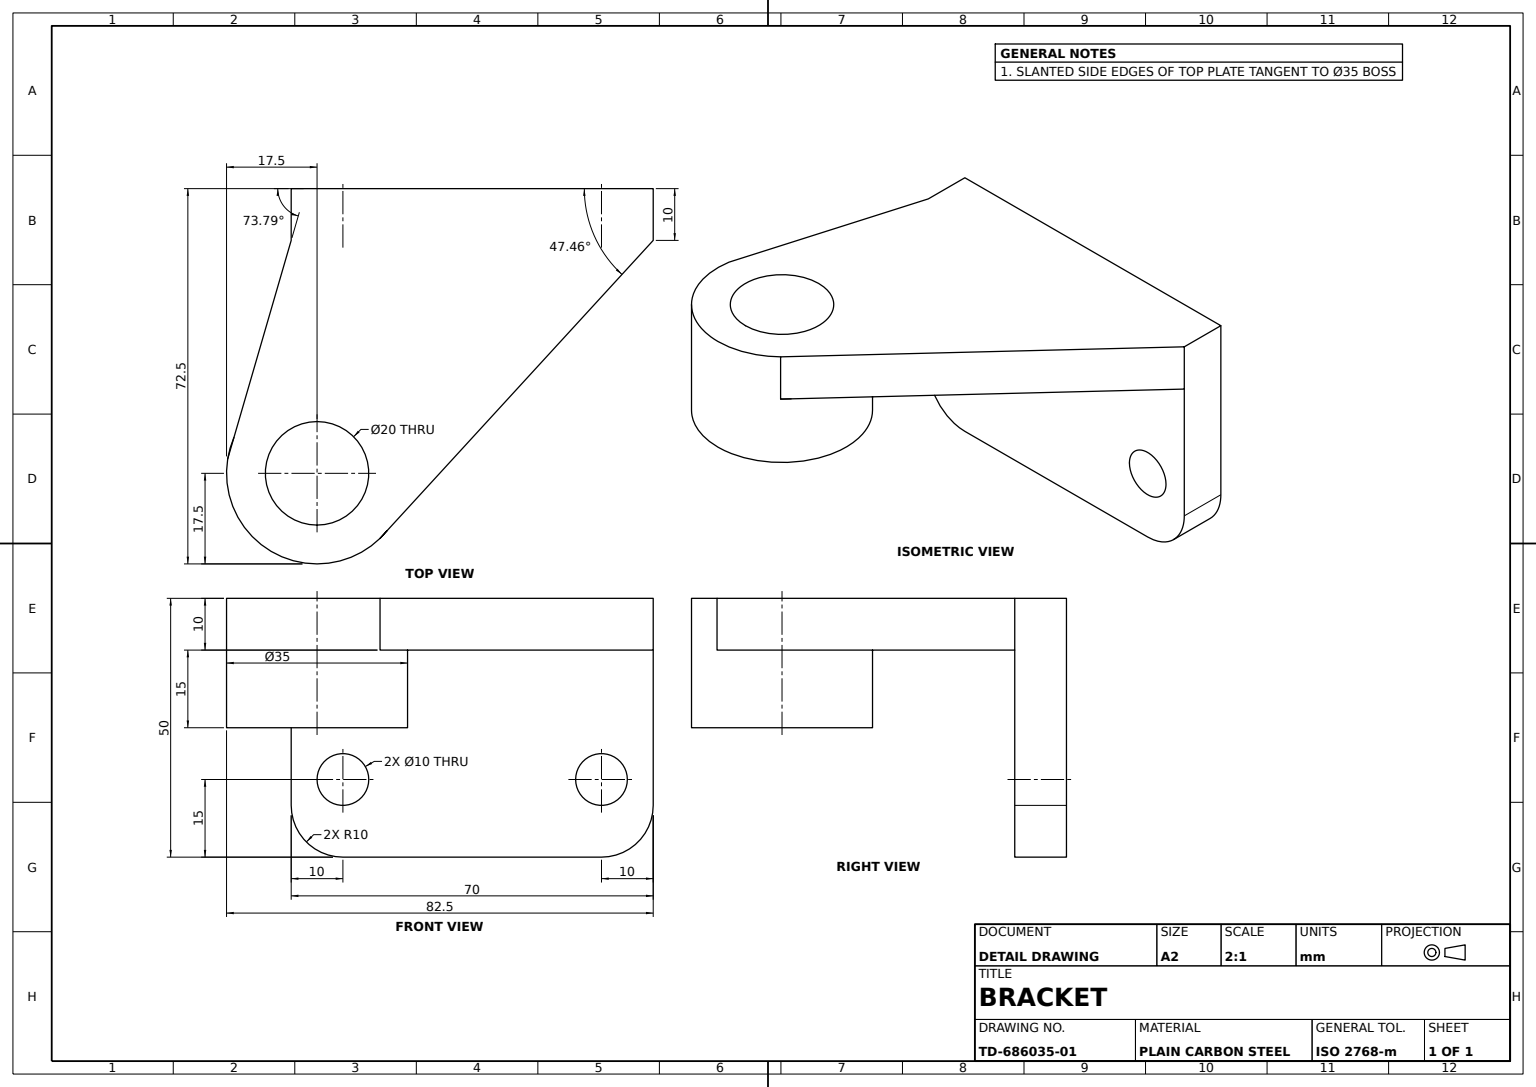
SolidWorks part; units mm, degrees
material "Plain Carbon Steel"
ref_plane "Front Plane" through (0, 0, 0) normal (0, 0, 1) x (1, 0, 0)
ref_plane "Top Plane" through (0, 0, 0) normal (0, 1, 0) x (1, 0, 0)
ref_plane "Right Plane" through (0, 0, 0) normal (1, 0, 0) x (0, 0, -1)
sketch "Base Plate Sketch" plane through (0, 0, 0) normal (0, 0, 1) x (1, 0, 0)
  line L0 (0, 0) -> (0, -40)
  line L3 (0, 0) -> (70, 0)
  line L4 (70, 0) -> (70, -40)
  line L6 (10, -50) -> (60, -50)
  arc A0 (0, -40) -> (10, -50) centre (10, -40) ccw
  arc A1 (60, -50) -> (70, -40) centre (60, -40) ccw
  dimension "D1" = 20
  dimension "D2" = 20
  dimension "D3" = 10
  dimension "D4" = 70
  dimension "D5" = 50
extrude "Base Plate" add sketch "Base Plate Sketch" along normal blind 10
sketch "Side Plate Sketch" plane through (0, 0, 0) normal (0, 1, 0) x (1, 0, 0)
  line L0 (70, -10) -> (17.1795, -67.5662)
  line L1 (0, -10) -> (0, 0) construction
  line L2 (0, -10) -> (-12.2787, -52.2259)
  line L3 (0, -10) -> (70, -10)
  line L4 (70, 0) -> (0, 0) construction
  circle A0 centre (5, -55) radius 17.5
  line M3 (0, -10) -> (70, -10)
  dimension "D1" = 35
  dimension "D2" = 35
  dimension "D3" = 5
  dimension "D4" = 17.1795
  dimension "D5" = 12.2787
  dimension "D6" = 52.2259
extrude "Side Plate" add sketch "Side Plate Sketch" against normal blind 10 contours A0 L0 L2 M3 | L0 A0 L2
sketch "Hub Boss Sketch" plane through (0, -10, 0) normal (0, -1, 0) x (1, 0, 0)
  circle A0 centre (5, 55) radius 17.5
  dimension "D1" = 35
  dimension "D2" = 35
extrude "Hub Boss Ø35" add sketch "Hub Boss Sketch" along normal blind 15
sketch "Hub Bore Sketch" plane through (0, -25, 0) normal (0, -1, 0) x (1, 0, 0)
  circle A0 centre (5, 55) radius 10
  dimension "D1" = 20
  dimension "D2" = 20
extrude "Hub Bore Ø20" cut sketch "Hub Bore Sketch" against normal blind 25
sketch "Side Plate Hole Sketch" plane through (0, 0, 10) normal (0, 0, 1) x (1, 0, 0)
  line L0 (70, -10) -> (18.5652, -10) construction
  line L1 (70, -40) -> (70, -10) construction
  line L2 (0, -10) -> (70, -10) construction
  line L3 (0, -10) -> (0, -40) construction
  circle A0 centre (10, -35) radius 5
  circle A1 centre (60, -35) radius 5
  dimension "D1" = 10
  dimension "D2" = 10
  dimension "D7" = 10
  dimension "D3" = 25
  dimension "D4" = 10
  dimension "D5" = 25
  dimension "D6" = 10
extrude "Side Plate Hole" cut sketch "Side Plate Hole Sketch" against normal blind 10
